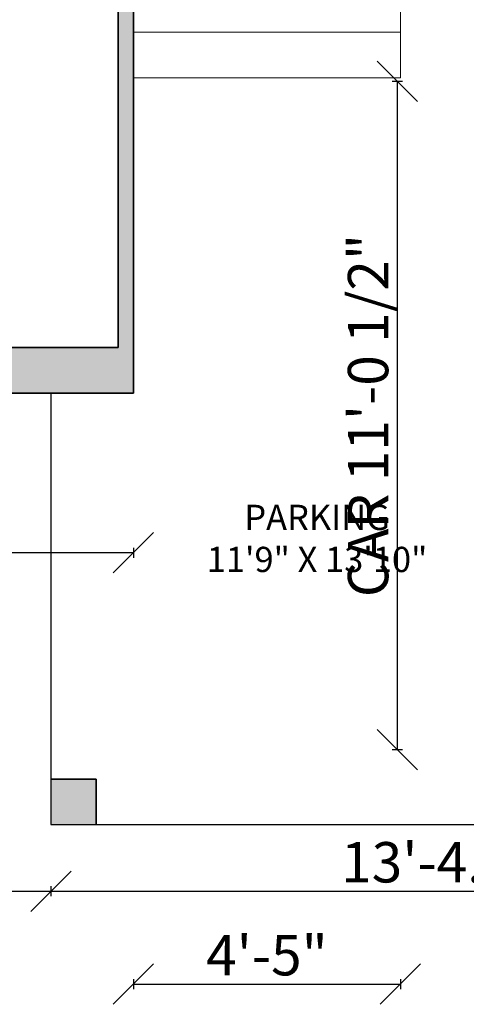
# Model space of a CAD drawing. Units: inches. Extents: x 2561 to 3163, y 493 to 1211.
# Tile 3 of 8: x 2943 to 3031, y 493 to 689. Entities that reach past the tile are written whole.
import ezdxf

# ---------------------------------------------------------------- set-up
doc = ezdxf.new("R2010")
doc.units = ezdxf.units.IN
for name, color, linetype, lineweight in [('A-ANNO-DIMS', 2, 'Continuous', 18), ('A-AREA-IDEN', 7, 'Continuous', 18), ('A-COLS', 7, 'Continuous', 35), ('A-COLS-PATT', 24, 'Continuous', 13), ('A-FLOR-STRS', 7, 'Continuous', 18), ('A-SITE-PRKG', 8, 'Continuous', 25), ('A-WALL', 7, 'Continuous', 35), ('A-WALL-PATT', 24, 'Continuous', 13)]:
    doc.layers.add(name, color=color, linetype=linetype, lineweight=lineweight)
doc.styles.get("Standard").update_dxf_attribs({"font": 'arial.ttf'})
doc.dimstyles.new('ISO-25', dxfattribs={"dimtxt": 8, "dimasz": 8, "dimexe": 1, "dimexo": 1, "dimtad": 1, "dimlunit": 3, "dimtxsty": 'Standard', "dimblk": 'OBLIQUE', "dimcen": 2.5, "dimadec": 0, "dimazin": 0, "dimtfac": 1, "dimtmove": 0, "dimatfit": 3, "dimfxl": 1, "dimfxlon": 1, "dimarcsym": 0})

# ---------------------------------------------------------------- blocks, each defined once
blk = doc.blocks.new('_Oblique')
at = {"color": 0, "linetype": 'ByBlock', "lineweight": -2}
blk.add_line((-0.5, -0.5), (0.5, 0.5), dxfattribs=at)
blk = doc.blocks.new('*D11')
at = {"layer": 'A-ANNO-DIMS', "color": 0, "lineweight": -2, "transparency": 16777216}
for p, q in [((3127.21, 695.07), (3129.21, 695.07)), ((3128.21, 695.07), (3128.21, 614.57)), ((3127.21, 614.57), (3129.21, 614.57))]:
    blk.add_line(p, q, dxfattribs=at)
at = {"layer": 'Defpoints', "color": 0, "transparency": 16777216}
for p in [(3109.27, 695.07), (2965.27, 614.57), (3128.21, 614.57)]:
    blk.add_point(p, dxfattribs=at)
at = {"layer": 'A-ANNO-DIMS', "color": 0, "lineweight": -2, "transparency": 16777216, "xscale": 8, "yscale": 8, "zscale": 8}
for p, rotation in [((3128.21, 695.07), 90), ((3128.21, 614.57), 270)]:
    blk.add_blockref('_Oblique', p, dxfattribs=dict(at, rotation=rotation))
at = {"layer": 'A-ANNO-DIMS', "color": 0, "transparency": 16777216, "insert": (3123.5, 654.82), "char_height": 8, "attachment_point": 5, "rotation": 90}
blk.add_mtext('6\'-8.5"', dxfattribs=at)
blk = doc.blocks.new('*D12')
at = {"layer": 'A-ANNO-DIMS', "color": 0, "lineweight": -2, "transparency": 16777216}
for p, q in [((3127.21, 614.57), (3129.21, 614.57)), ((3128.21, 614.57), (3128.21, 529.07)), ((3127.21, 529.07), (3129.21, 529.07))]:
    blk.add_line(p, q, dxfattribs=at)
at = {"layer": 'Defpoints', "color": 0, "transparency": 16777216}
for p in [(2965.27, 614.57), (2965.27, 529.07), (3128.21, 529.07)]:
    blk.add_point(p, dxfattribs=at)
at = {"layer": 'A-ANNO-DIMS', "color": 0, "lineweight": -2, "transparency": 16777216, "xscale": 8, "yscale": 8, "zscale": 8}
for p, rotation in [((3128.21, 614.57), 90), ((3128.21, 529.07), 270)]:
    blk.add_blockref('_Oblique', p, dxfattribs=dict(at, rotation=rotation))
at = {"layer": 'A-ANNO-DIMS', "color": 0, "transparency": 16777216, "insert": (3123.5, 571.82), "char_height": 8, "attachment_point": 5, "rotation": 90}
blk.add_mtext('7\'-1.5"', dxfattribs=at)
blk = doc.blocks.new('*D14')
at = {"layer": 'A-ANNO-DIMS', "color": 0, "lineweight": -2, "transparency": 16777216}
for p, q in [((2948.92, 516.82), (2948.92, 514.82)), ((2948.92, 515.82), (3109.27, 515.82)), ((3109.27, 516.82), (3109.27, 514.82))]:
    blk.add_line(p, q, dxfattribs=at)
at = {"layer": 'Defpoints', "color": 0, "transparency": 16777216}
for p in [(2948.92, 529.07), (3109.27, 529.07), (3109.27, 515.82)]:
    blk.add_point(p, dxfattribs=at)
at = {"layer": 'A-ANNO-DIMS', "color": 0, "lineweight": -2, "transparency": 16777216, "xscale": 8, "yscale": 8, "zscale": 8, "rotation": 180}
blk.add_blockref('_Oblique', (2948.92, 515.82), dxfattribs=at)
at = {"layer": 'A-ANNO-DIMS', "color": 0, "lineweight": -2, "transparency": 16777216, "xscale": 8, "yscale": 8, "zscale": 8}
blk.add_blockref('_Oblique', (3109.27, 515.82), dxfattribs=at)
at = {"layer": 'A-ANNO-DIMS', "color": 0, "transparency": 16777216, "insert": (3029.1, 520.53), "char_height": 8, "attachment_point": 5}
blk.add_mtext('13\'-4.36"', dxfattribs=at)
blk = doc.blocks.new('*D15')
at = {"layer": 'A-ANNO-DIMS', "color": 0, "lineweight": -2, "transparency": 16777216}
for p, q in [((2629.27, 516.82), (2629.27, 514.82)), ((2629.27, 515.82), (2948.92, 515.82)), ((2948.92, 516.82), (2948.92, 514.82))]:
    blk.add_line(p, q, dxfattribs=at)
at = {"layer": 'Defpoints', "color": 0, "transparency": 16777216}
for p in [(2629.27, 614.57), (2948.92, 614.57), (2948.92, 515.82)]:
    blk.add_point(p, dxfattribs=at)
at = {"layer": 'A-ANNO-DIMS', "color": 0, "lineweight": -2, "transparency": 16777216, "xscale": 8, "yscale": 8, "zscale": 8, "rotation": 180}
blk.add_blockref('_Oblique', (2629.27, 515.82), dxfattribs=at)
at = {"layer": 'A-ANNO-DIMS', "color": 0, "lineweight": -2, "transparency": 16777216, "xscale": 8, "yscale": 8, "zscale": 8}
blk.add_blockref('_Oblique', (2948.92, 515.82), dxfattribs=at)
at = {"layer": 'A-ANNO-DIMS', "color": 0, "transparency": 16777216, "insert": (2789.1, 520.53), "char_height": 8, "attachment_point": 5}
blk.add_mtext('26\'-7.64"', dxfattribs=at)
blk = doc.blocks.new('*D17')
at = {"layer": 'A-ANNO-DIMS', "color": 0, "lineweight": -2, "transparency": 16777216}
for p, q in [((2571.63, 1093.07), (2569.63, 1093.07)), ((2570.63, 1093.07), (2570.63, 529.07)), ((2571.63, 529.07), (2569.63, 529.07))]:
    blk.add_line(p, q, dxfattribs=at)
at = {"layer": 'Defpoints', "color": 0, "transparency": 16777216}
for p in [(2629.27, 1093.07), (2570.63, 529.07), (3109.27, 529.07)]:
    blk.add_point(p, dxfattribs=at)
at = {"layer": 'A-ANNO-DIMS', "color": 0, "lineweight": -2, "transparency": 16777216, "xscale": 8, "yscale": 8, "zscale": 8}
for p, rotation in [((2570.63, 1093.07), 90), ((2570.63, 529.07), 270)]:
    blk.add_blockref('_Oblique', p, dxfattribs=dict(at, rotation=rotation))
at = {"layer": 'A-ANNO-DIMS', "color": 0, "transparency": 16777216, "insert": (2566, 811.07), "char_height": 8, "attachment_point": 5, "rotation": 90}
blk.add_mtext("47'", dxfattribs=at)
blk = doc.blocks.new('*D20')
at = {"layer": 'A-ANNO-DIMS', "color": 0, "lineweight": -2, "transparency": 16777216}
for p, q in [((3018.58, 676.33), (3016.58, 676.33)), ((3017.58, 543.86), (3017.58, 676.33)), ((3018.58, 543.86), (3016.58, 543.86))]:
    blk.add_line(p, q, dxfattribs=at)
at = {"layer": 'Defpoints', "color": 0, "transparency": 16777216}
for p in [(3017.58, 676.33), (3037.45, 676.33), (3037.45, 543.86)]:
    blk.add_point(p, dxfattribs=at)
at = {"layer": 'A-ANNO-DIMS', "color": 0, "lineweight": -2, "transparency": 16777216, "xscale": 8, "yscale": 8, "zscale": 8}
for p, rotation in [((3017.58, 676.33), 90), ((3017.58, 543.86), 270)]:
    blk.add_blockref('_Oblique', p, dxfattribs=dict(at, rotation=rotation))
at = {"layer": 'A-ANNO-DIMS', "color": 0, "transparency": 16777216, "insert": (3012.82, 610.1), "char_height": 8, "attachment_point": 5, "rotation": 90}
blk.add_mtext('CAR 11\'-0 1/2"', dxfattribs=at)
blk = doc.blocks.new('*D32')
at = {"layer": 'A-ANNO-DIMS', "color": 0, "lineweight": -2, "transparency": 16777216}
for p, q in [((2965.27, 498.42), (2965.27, 496.42)), ((3018.2, 498.42), (3018.2, 496.42)), ((2965.27, 497.42), (3018.2, 497.42))]:
    blk.add_line(p, q, dxfattribs=at)
at = {"layer": 'Defpoints', "color": 0, "transparency": 16777216}
for p in [(2965.27, 677.07), (3018.2, 677.07), (3018.2, 497.42)]:
    blk.add_point(p, dxfattribs=at)
at = {"layer": 'A-ANNO-DIMS', "color": 0, "lineweight": -2, "transparency": 16777216, "xscale": 8, "yscale": 8, "zscale": 8, "rotation": 180}
blk.add_blockref('_Oblique', (2965.27, 497.42), dxfattribs=at)
at = {"layer": 'A-ANNO-DIMS', "color": 0, "lineweight": -2, "transparency": 16777216, "xscale": 8, "yscale": 8, "zscale": 8}
blk.add_blockref('_Oblique', (3018.2, 497.42), dxfattribs=at)
at = {"layer": 'A-ANNO-DIMS', "color": 0, "transparency": 16777216, "insert": (2991.73, 502.11), "char_height": 8, "attachment_point": 5}
blk.add_mtext('4\'-5"', dxfattribs=at)
blk = doc.blocks.new('*D64')
at = {"layer": 'A-ANNO-DIMS', "color": 0, "lineweight": -2, "transparency": 16777216}
for p, q in [((2936.56, 583.92), (2936.56, 581.92)), ((2965.27, 583.92), (2965.27, 581.92)), ((2936.56, 582.92), (2887.27, 582.92)), ((2965.27, 582.92), (2936.56, 582.92))]:
    blk.add_line(p, q, dxfattribs=at)
at = {"layer": 'Defpoints', "color": 0, "transparency": 16777216}
for p in [(2936.56, 614.57), (2965.27, 614.57), (2936.56, 582.92)]:
    blk.add_point(p, dxfattribs=at)
at = {"layer": 'A-ANNO-DIMS', "color": 0, "lineweight": -2, "transparency": 16777216, "xscale": 8, "yscale": 8, "zscale": 8, "rotation": 180}
blk.add_blockref('_Oblique', (2936.56, 582.92), dxfattribs=at)
at = {"layer": 'A-ANNO-DIMS', "color": 0, "lineweight": -2, "transparency": 16777216, "xscale": 8, "yscale": 8, "zscale": 8}
blk.add_blockref('_Oblique', (2965.27, 582.92), dxfattribs=at)
at = {"layer": 'A-ANNO-DIMS', "color": 0, "transparency": 16777216, "insert": (2907.92, 587.68), "char_height": 8, "attachment_point": 5}
blk.add_mtext('2\'-4 1/2"', dxfattribs=at)

msp = doc.modelspace()

# ---------------------------------------------------------------- hatches: boundary and pattern name
at = {"layer": 'A-COLS-PATT'}
h = msp.add_hatch(color=256, dxfattribs=at)
h.dxf.hatch_style = 1
h.paths.add_polyline_path([(3109.274, 538.069), (3100.274, 538.069), (3100.274, 529.069), (3109.274, 529.069)])
h.paths.add_polyline_path([(2957.918, 538.069), (2948.918, 538.069), (2948.918, 529.069), (2957.918, 529.069)])
at = {"layer": 'A-WALL-PATT'}
h = msp.add_hatch(color=256, dxfattribs=at)
h.dxf.hatch_style = 1
h.paths.add_polyline_path([(2665.022, 1093.069), (2629.274, 1093.069), (2629.274, 1056.034), (2638.274, 1056.034), (2638.274, 1084.069), (2665.022, 1084.069)])
h.paths.add_polyline_path([(2785.37, 1093.069), (2727.193, 1093.069), (2727.193, 1084.069), (2773.274, 1084.069), (2773.274, 940.069), (2762.774, 940.069), (2762.774, 935.569), (2777.774, 935.569), (2777.774, 971.569), (2825.774, 971.569), (2825.774, 935.569), (2921.774, 935.569), (2921.774, 940.069), (2830.274, 940.069), (2830.274, 976.069), (2777.774, 976.069), (2777.774, 1084.069), (2785.37, 1084.069)])
h.paths.add_polyline_path([(2856.568, 1093.069), (2816.168, 1093.069), (2816.168, 1084.069), (2825.774, 1084.069), (2825.774, 1008.069), (2830.274, 1008.069), (2830.274, 1084.069), (2856.568, 1084.069)], flags=17)
h.paths.add_polyline_path([(3006.866, 1093.069), (2929.24, 1093.069), (2929.24, 1084.069), (2962.274, 1084.069), (2962.274, 940.069), (2957.774, 940.069), (2957.774, 935.569), (2970.774, 935.569), (2970.774, 940.069), (2968.274, 940.069), (2968.274, 1084.069), (3006.866, 1084.069)])
h.paths.add_polyline_path([(3109.274, 1093.069), (3068.804, 1093.069), (3068.804, 1084.069), (3100.274, 1084.069), (3100.274, 1061.194), (3109.274, 1061.194)])
h.paths.add_polyline_path([(3109.274, 991.723), (3100.274, 991.723), (3100.274, 940.069), (3010.774, 940.069), (3010.774, 935.569), (3010.774, 911.569), (3015.274, 911.569), (3015.274, 935.569), (3100.274, 935.569), (3100.274, 927.07), (3109.274, 927.07)])
h.paths.add_polyline_path([(3109.274, 897.327), (3100.274, 897.327), (3100.274, 881.569), (2957.774, 881.569), (2957.774, 872.569), (3100.274, 872.569), (3100.274, 805.791), (3109.274, 805.791)])
h.paths.add_polyline_path([(2638.274, 982.372), (2629.274, 982.372), (2629.274, 927.027), (2638.274, 927.027), (2638.274, 935.569), (2722.274, 935.569), (2722.274, 919.569), (2726.774, 919.569), (2726.774, 940.069), (2638.274, 940.069)])
h.paths.add_polyline_path([(2638.274, 883.069), (2726.774, 883.069), (2726.774, 887.569), (2638.274, 887.569), (2638.274, 897.75), (2629.274, 897.75), (2629.274, 856.591), (2638.274, 856.591)])
h.paths.add_polyline_path([(2726.774, 851.069), (2722.274, 851.069), (2722.274, 772.069), (2638.274, 772.069), (2638.274, 802.178), (2629.274, 802.178), (2629.274, 725.136), (2638.274, 725.136), (2638.274, 767.569), (2726.774, 767.569)])
h.paths.add_polyline_path([(2638.274, 659.235), (2629.274, 659.235), (2629.274, 614.569), (2638.274, 614.569)])
h.paths.add_polyline_path([(2664.613, 623.569), (2638.274, 623.569), (2638.274, 614.569), (2664.613, 614.569)])
h.paths.add_polyline_path([(2787.908, 623.569), (2777.774, 623.569), (2777.774, 767.569), (2825.774, 767.569), (2825.774, 659.569), (2830.274, 659.569), (2830.274, 767.569), (2836.774, 767.569), (2836.774, 772.069), (2766.674, 772.069), (2766.674, 767.569), (2773.274, 767.569), (2773.274, 623.569), (2722.435, 623.569), (2722.435, 614.569), (2787.908, 614.569)])
h.paths.add_polyline_path([(2883.664, 623.569), (2867.474, 623.569), (2818.294, 623.569), (2818.294, 614.569), (2883.664, 614.569)])
h.paths.add_polyline_path([(2965.274, 772.069), (2872.774, 772.069), (2872.774, 767.569), (2962.274, 767.569), (2962.274, 623.569), (2936.565, 623.569), (2936.565, 614.569), (2965.274, 614.569)])
h.paths.add_polyline_path([(3109.274, 758.846), (3100.274, 758.846), (3100.274, 701.069), (3013.274, 701.069), (3013.274, 695.069), (3109.274, 695.069)])
h.paths.add_polyline_path([(2965.274, 824.569), (2957.774, 824.569), (2957.774, 772.069), (2965.274, 772.069)])

# ---------------------------------------------------------------- linework, layer by layer
at = {"layer": 'A-COLS'}
for p, q in [((2957.918, 538.069), (2948.918, 538.069)), ((2957.918, 529.069), (2957.918, 538.069))]:
    msp.add_line(p, q, dxfattribs=at)
at = {"layer": 'A-FLOR-STRS'}
for p, q in [((3018.195, 695.069), (3018.195, 677.069)), ((3018.195, 686.069), (2965.274, 686.069)), ((3018.195, 677.069), (2965.274, 677.069))]:
    msp.add_line(p, q, dxfattribs=at)
at = {"layer": 'A-SITE-PRKG'}
for p, q in [((2948.918, 614.569), (2948.918, 529.069)), ((2948.918, 529.069), (3109.274, 529.069))]:
    msp.add_line(p, q, dxfattribs=at)
at = {"layer": 'A-WALL'}
for p, q in [((2965.274, 614.569), (2965.274, 772.069)), ((2962.274, 623.569), (2962.274, 767.569)), ((2962.274, 623.569), (2777.774, 623.569))]:
    msp.add_line(p, q, dxfattribs=at)
msp.add_lwpolyline([(3109.274, 695.069), (3109.274, 1093.069), (2629.274, 1093.069), (2629.274, 614.569), (2965.274, 614.569)], dxfattribs=at)

# ---------------------------------------------------------------- texts
at = {"layer": 'A-AREA-IDEN', "insert": (2971.048, 592.425), "char_height": 5, "attachment_point": 1}
msp.add_mtext_dynamic_manual_height_columns('\\pxqc;PARKING\\P11\'9" X 13\'10"', width=61.24894, gutter_width=12.5, heights=[0], dxfattribs=at)

# ---------------------------------------------------------------- dimensions: what is measured, and where the dimension line sits
at = {"layer": 'A-ANNO-DIMS'}
for base, p1, p2, angle, override, picture, middle in [((2570.627, 529.069), (2629.274, 1093.069), (3109.274, 529.069), 90, {"dimclrd": 0, "dimclre": 0, "dimclrt": 0}, '*D17', (2566.002, 811.069)), ((3128.213, 614.569), (3109.274, 695.069), (2965.274, 614.569), 90, {"dimclrd": 0, "dimclre": 0, "dimclrt": 0, "dimtmove": 1}, '*D11', (3123.503, 654.819)), ((3128.213, 529.069), (2965.274, 614.569), (2965.274, 529.069), 90, {"dimclrd": 0, "dimclre": 0, "dimclrt": 0, "dimtmove": 1}, '*D12', (3123.503, 571.819)), ((2936.565, 582.919), (2965.274, 614.569), (2936.565, 614.569), 180, {"dimdec": 1, "dimlfac": 1, "dimrnd": 0, "dimzin": 1, "dimdsep": 46, "dimlunit": 4, "dimfrac": 2}, '*D64', (2907.918, 587.68))]:
    dim = msp.add_linear_dim(base=base, p1=p1, p2=p2, angle=angle, dimstyle='ISO-25', override=override, dxfattribs=at)
    dim.commit()
    dim.dimension.update_dxf_attribs({"geometry": picture, "text_midpoint": middle})
dim = msp.add_linear_dim(base=(3017.58, 676.333), p1=(3037.451, 543.862), p2=(3037.451, 676.333), angle=90, text='CAR <>', dimstyle='ISO-25', override={"dimdec": 1, "dimlfac": 1, "dimrnd": 0, "dimzin": 1, "dimdsep": 46, "dimlunit": 4, "dimfrac": 2}, dxfattribs=at)
dim.commit()
dim.dimension.update_dxf_attribs({"geometry": '*D20', "text_midpoint": (3012.819, 610.098)})
for base, p1, p2, override, picture, middle in [((3018.195, 497.419), (2965.274, 677.069), (3018.195, 677.069), {"dimdec": 1, "dimlfac": 1, "dimrnd": 0, "dimzin": 1, "dimdsep": 46, "dimlunit": 4, "dimfrac": 2}, '*D32', (2991.735, 502.112)), ((2948.918, 515.818), (2629.274, 614.569), (2948.918, 614.569), {"dimclrd": 0, "dimclre": 0, "dimclrt": 0}, '*D15', (2789.096, 520.527)), ((3109.274, 515.818), (2948.918, 529.069), (3109.274, 529.069), {"dimclrd": 0, "dimclre": 0, "dimclrt": 0}, '*D14', (3029.096, 520.53))]:
    dim = msp.add_linear_dim(base=base, p1=p1, p2=p2, dimstyle='ISO-25', override=override, dxfattribs=at)
    dim.commit()
    dim.dimension.update_dxf_attribs({"geometry": picture, "text_midpoint": middle})

doc.saveas('drawing.dxf')
